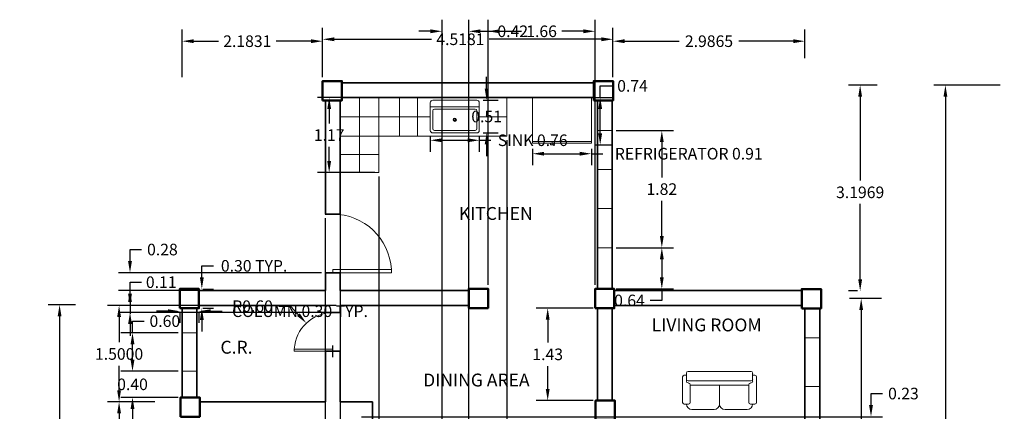
# Model space of a CAD drawing. Units: metres. Extents: x 473.2 to 488.6, y 701.8 to 717.3.
# Tile 4 of 4: x 473.3 to 488.6, y 711.3 to 717.3. Entities that reach past the tile are written whole.
import ezdxf

# ---------------------------------------------------------------- set-up
doc = ezdxf.new("R2010")
doc.units = ezdxf.units.M
doc.header["$PDMODE"] = 32
for name, color, linetype, lineweight in [('A-ANNO-DIMS', 2, 'Continuous', 18), ('A-AREA-IDEN', 7, 'Continuous', 18), ('A-COLS', 7, 'Continuous', 50), ('A-DOOR', 3, 'Continuous', 18), ('A-EQPM', 8, 'Continuous', 18), ('A-FLOR-CASE', 9, 'Continuous', 18), ('A-FLOR-FIXT', 9, 'Continuous', 18), ('A-FURN', 8, 'Continuous', 18), ('A-GLAZ', 4, 'Continuous', 18), ('A-WALL', 7, 'Continuous', 35)]:
    doc.layers.add(name, color=color, linetype=linetype, lineweight=lineweight)
doc.styles.get("Standard").update_dxf_attribs({"font": 'arial.ttf'})
doc.dimstyles.get("Standard").update_dxf_attribs({"dimtxt": 0.18, "dimasz": 0.18, "dimexe": 0.18, "dimexo": 0.0625, "dimgap": 0.09, "dimtad": 0, "dimtih": 1, "dimtoh": 1, "dimdec": 4, "dimzin": 0, "dimdsep": 46, "dimtxsty": 'Standard', "dimcen": 0.09, "dimadec": 0, "dimazin": 0, "dimtfac": 1, "dimtdec": 4, "dimtofl": 0, "dimtmove": 0, "dimatfit": 3, "dimfxl": 1, "dimtolj": 1, "dimtzin": 0, "dimarcsym": 0})

# ---------------------------------------------------------------- blocks, each defined once
blk = doc.blocks.new('A$C02A636C4')
for p, q in [((0, 0.572), (0, 0.126)), ((0.068, 0.601), (0.029, 0.601)), ((0.068, 0.64), (0.068, 0.601)), ((0.068, 0.533), (0.068, 0.601)), ((0.068, 0.495), (0.068, 0.543)), ((1.203, 0.669), (0.097, 0.669)), ((1.232, 0.64), (1.232, 0.601)), ((1.232, 0.601), (1.271, 0.601)), ((1.232, 0.533), (1.232, 0.601)), ((1.232, 0.495), (1.232, 0.543)), ((1.3, 0.572), (1.3, 0.126)), ((1.203, 0.504), (0.097, 0.504)), ((0.107, 0.466), (0.097, 0.466)), ((0.136, 0.126), (0.136, 0.436)), ((1.164, 0.427), (0.136, 0.427)), ((0.65, 0.097), (0.65, 0.427)), ((1.164, 0.126), (1.164, 0.436)), ((1.193, 0.466), (1.203, 0.466)), ((0.029, 0.097), (0.107, 0.097)), ((0.165, 0), (0.553, 0)), ((0.747, 0), (1.135, 0)), ((1.271, 0.097), (1.193, 0.097))]:
    blk.add_line(p, q)
for centre, radius, start, end in [((0.029, 0.572), 0.0291, 90, 180), ((0.097, 0.64), 0.0291, 90, 180), ((0.097, 0.533), 0.0291, 180, 270), ((1.203, 0.64), 0.0291, 0, 90), ((1.203, 0.533), 0.0291, 270, 0), ((1.271, 0.572), 0.0291, 0, 90), ((0.097, 0.495), 0.0291, 180, 270), ((0.107, 0.436), 0.0291, 0, 90), ((1.193, 0.436), 0.0291, 90, 180), ((1.203, 0.495), 0.0291, 270, 0), ((0.029, 0.126), 0.0291, 180, 270), ((0.165, 0.097), 0.097, 180, 270), ((0.107, 0.126), 0.0291, 270, 0), ((0.553, 0.097), 0.097, 270, 0), ((0.747, 0.097), 0.097, 180, 270), ((1.135, 0.097), 0.097, 270, 0), ((1.193, 0.126), 0.0291, 180, 270), ((1.271, 0.126), 0.0291, 270, 0)]:
    blk.add_arc(centre, radius, start, end)
blk = doc.blocks.new('Sink-single - 30 in top')
blk.add_line((-15, -3.999996), (15, -3.999996))
for points in [[(-13.5, 0), (13.5, 0)], [(-15, -18.499996), (-15, -1.5)], [(-12.5, -5.499996), (12.5, -5.499996)], [(15, -1.5), (15, -18.499996)], [(-13.5, -17.499996), (-13.5, -6.499996)], [(13.5, -6.499996), (13.5, -17.499996)], [(13.5, -19.999996), (-13.5, -19.999996)], [(12.5, -18.499996), (-12.5, -18.499996)]]:
    blk.add_lwpolyline(points)
for radius in [1, 0.5]:
    blk.add_circle((0, -11.999996), radius)
for centre, radius, start, end in [((-13.5, -1.5), 1.5, 90, 180), ((-12.5, -6.499996), 1, 90, 180), ((12.5, -6.499996), 1, 0, 90), ((13.5, -1.5), 1.5, 0, 90), ((-12.5, -17.499996), 1, 180, 270), ((12.5, -17.499996), 1, 270, 0), ((-13.5, -18.499996), 1.5, 180, 270), ((13.5, -18.499996), 1.5, 270, 0)]:
    blk.add_arc(centre, radius, start, end)
blk = doc.blocks.new('Refrigerator-2 door - 36 in top')
for p, q in [((0, -26.999999), (36, -26.999999)), ((11, -27.999999), (11, -28.999999)), ((11, -28.999999), (13, -28.999999)), ((12, -26.999999), (12, -28.999999)), ((13, -28.999999), (13, -27.999999))]:
    blk.add_line(p, q)
blk.add_lwpolyline([(0, -27.999999), (0, 0), (36, 0), (36, -27.999999)], close=True)
blk = doc.blocks.new('*D6')
at = {"layer": 'A-ANNO-DIMS', "color": 0, "lineweight": -2, "transparency": 16777216}
for p, q in [((482.501, 716.452), (482.501, 717.189)), ((485.488, 716.744), (485.488, 717.189)), ((482.681, 717.009), (483.529, 717.009)), ((485.308, 717.009), (484.461, 717.009))]:
    blk.add_line(p, q, dxfattribs=at)
at = {"layer": 'A-ANNO-DIMS', "color": 0, "transparency": 16777216}
for points in [[(482.681, 717.039), (482.681, 716.979), (482.501, 717.009)], [(485.308, 717.039), (485.308, 716.979), (485.488, 717.009)]]:
    blk.add_solid(points, dxfattribs=at)
at = {"layer": 'Defpoints', "color": 0, "transparency": 16777216}
for p in [(485.488, 717.009), (485.488, 716.681), (482.501, 716.39)]:
    blk.add_point(p, dxfattribs=at)
at = {"layer": 'A-ANNO-DIMS', "color": 0, "transparency": 16777216, "insert": (483.995, 717.009), "char_height": 0.18, "width": 1.24026, "attachment_point": 5}
blk.add_mtext('\\A1;2.9865', dxfattribs=at)
blk = doc.blocks.new('*D7')
at = {"layer": 'A-ANNO-DIMS', "color": 0, "lineweight": -2, "transparency": 16777216}
for p, q in [((477.983, 716.452), (477.983, 717.219)), ((482.501, 716.644), (482.501, 717.219)), ((478.163, 717.039), (479.677, 717.039)), ((482.321, 717.039), (480.577, 717.039))]:
    blk.add_line(p, q, dxfattribs=at)
at = {"layer": 'A-ANNO-DIMS', "color": 0, "transparency": 16777216}
for points in [[(478.163, 717.069), (478.163, 717.009), (477.983, 717.039)], [(482.321, 717.069), (482.321, 717.009), (482.501, 717.039)]]:
    blk.add_solid(points, dxfattribs=at)
at = {"layer": 'Defpoints', "color": 0, "transparency": 16777216}
for p in [(482.501, 717.039), (482.501, 716.581), (477.983, 716.39)]:
    blk.add_point(p, dxfattribs=at)
at = {"layer": 'A-ANNO-DIMS', "color": 0, "transparency": 16777216, "insert": (480.127, 717.039), "char_height": 0.18, "width": 1.24026, "attachment_point": 5}
blk.add_mtext('\\A1;4.5181', dxfattribs=at)
blk = doc.blocks.new('*D8')
at = {"layer": 'A-ANNO-DIMS', "color": 0, "lineweight": -2, "transparency": 16777216}
for p, q in [((475.798, 716.452), (475.798, 717.189)), ((477.981, 716.744), (477.981, 717.189)), ((475.978, 717.009), (476.363, 717.009)), ((477.801, 717.009), (477.259, 717.009))]:
    blk.add_line(p, q, dxfattribs=at)
at = {"layer": 'A-ANNO-DIMS', "color": 0, "transparency": 16777216}
for points in [[(475.978, 717.039), (475.978, 716.979), (475.798, 717.009)], [(477.801, 717.039), (477.801, 716.979), (477.981, 717.009)]]:
    blk.add_solid(points, dxfattribs=at)
at = {"layer": 'Defpoints', "color": 0, "transparency": 16777216}
for p in [(477.981, 717.009), (477.981, 716.681), (475.798, 716.39)]:
    blk.add_point(p, dxfattribs=at)
at = {"layer": 'A-ANNO-DIMS', "color": 0, "transparency": 16777216, "insert": (476.811, 717.009), "char_height": 0.18, "width": 1.24026, "attachment_point": 5}
blk.add_mtext('\\A1;2.1831', dxfattribs=at)
blk = doc.blocks.new('*D10')
at = {"layer": 'A-ANNO-DIMS', "color": 0, "lineweight": -2, "transparency": 16777216}
for p, q in [((475.082, 712.905), (474.636, 712.905)), ((474.816, 712.725), (474.816, 712.332)), ((474.816, 711.585), (474.816, 711.968)), ((475.373, 711.405), (474.636, 711.405))]:
    blk.add_line(p, q, dxfattribs=at)
at = {"layer": 'A-ANNO-DIMS', "color": 0, "transparency": 16777216}
for points in [[(474.786, 712.725), (474.846, 712.725), (474.816, 712.905)], [(474.786, 711.585), (474.846, 711.585), (474.816, 711.405)]]:
    blk.add_solid(points, dxfattribs=at)
at = {"layer": 'Defpoints', "color": 0, "transparency": 16777216}
for p in [(474.816, 712.905), (475.144, 712.905), (475.435, 711.405)]:
    blk.add_point(p, dxfattribs=at)
at = {"layer": 'A-ANNO-DIMS', "color": 0, "transparency": 16777216, "insert": (474.816, 712.15), "char_height": 0.18, "width": 1.24026, "attachment_point": 5}
blk.add_mtext('\\A1;1.5000', dxfattribs=at)
blk = doc.blocks.new('*D11')
at = {"layer": 'A-ANNO-DIMS', "color": 0, "lineweight": -2, "transparency": 16777216}
for p, q in [((475.082, 711.405), (474.636, 711.405)), ((474.816, 711.225), (474.816, 709.784)), ((474.816, 707.857), (474.816, 709.421)), ((475.373, 707.677), (474.636, 707.677))]:
    blk.add_line(p, q, dxfattribs=at)
at = {"layer": 'A-ANNO-DIMS', "color": 0, "transparency": 16777216}
for points in [[(474.786, 711.225), (474.846, 711.225), (474.816, 711.405)], [(474.786, 707.857), (474.846, 707.857), (474.816, 707.677)]]:
    blk.add_solid(points, dxfattribs=at)
at = {"layer": 'Defpoints', "color": 0, "transparency": 16777216}
for p in [(474.816, 711.405), (475.144, 711.405), (475.435, 707.677)]:
    blk.add_point(p, dxfattribs=at)
at = {"layer": 'A-ANNO-DIMS', "color": 0, "transparency": 16777216, "insert": (474.816, 709.602), "char_height": 0.18, "width": 1.24026, "attachment_point": 5}
blk.add_mtext('\\A1;3.7277', dxfattribs=at)
blk = doc.blocks.new('*D13')
at = {"layer": 'A-ANNO-DIMS', "color": 0, "lineweight": -2, "transparency": 16777216}
for p, q in [((474.139, 712.914), (473.71, 712.914)), ((473.89, 712.734), (473.89, 708.817)), ((473.89, 704.612), (473.89, 708.453)), ((473.889, 704.432), (473.71, 704.432))]:
    blk.add_line(p, q, dxfattribs=at)
at = {"layer": 'A-ANNO-DIMS', "color": 0, "transparency": 16777216}
for points in [[(473.86, 712.734), (473.92, 712.734), (473.89, 712.914)], [(473.86, 704.612), (473.92, 704.612), (473.89, 704.432)]]:
    blk.add_solid(points, dxfattribs=at)
at = {"layer": 'Defpoints', "color": 0, "transparency": 16777216}
for p in [(473.89, 712.914), (474.201, 712.914), (473.952, 704.432)]:
    blk.add_point(p, dxfattribs=at)
at = {"layer": 'A-ANNO-DIMS', "color": 0, "transparency": 16777216, "insert": (473.89, 708.635), "char_height": 0.18, "width": 1.24026, "attachment_point": 5}
blk.add_mtext('\\A1;8.4814', dxfattribs=at)
blk = doc.blocks.new('*D14')
at = {"layer": 'A-ANNO-DIMS', "color": 0, "lineweight": -2, "transparency": 16777216}
for p, q in [((486.68, 713.013), (486.183, 713.013)), ((486.363, 712.833), (486.363, 710.74)), ((486.363, 707.857), (486.363, 710.376)), ((486.92, 707.677), (486.183, 707.677))]:
    blk.add_line(p, q, dxfattribs=at)
at = {"layer": 'A-ANNO-DIMS', "color": 0, "transparency": 16777216}
for points in [[(486.333, 712.833), (486.393, 712.833), (486.363, 713.013)], [(486.333, 707.857), (486.393, 707.857), (486.363, 707.677)]]:
    blk.add_solid(points, dxfattribs=at)
at = {"layer": 'Defpoints', "color": 0, "transparency": 16777216}
for p in [(486.363, 713.013), (486.743, 713.013), (486.982, 707.677)]:
    blk.add_point(p, dxfattribs=at)
at = {"layer": 'A-ANNO-DIMS', "color": 0, "transparency": 16777216, "insert": (486.363, 710.558), "char_height": 0.18, "width": 1.24026, "attachment_point": 5}
blk.add_mtext('\\A1;5.3358', dxfattribs=at)
blk = doc.blocks.new('*D16')
at = {"layer": 'A-ANNO-DIMS', "color": 0, "lineweight": -2, "transparency": 16777216}
for p, q in [((486.612, 716.326), (486.167, 716.326)), ((486.347, 716.146), (486.347, 714.843)), ((486.347, 713.309), (486.347, 714.48)), ((486.308, 713.129), (486.167, 713.129))]:
    blk.add_line(p, q, dxfattribs=at)
at = {"layer": 'A-ANNO-DIMS', "color": 0, "transparency": 16777216}
for points in [[(486.317, 716.146), (486.377, 716.146), (486.347, 716.326)], [(486.317, 713.309), (486.377, 713.309), (486.347, 713.129)]]:
    blk.add_solid(points, dxfattribs=at)
at = {"layer": 'Defpoints', "color": 0, "transparency": 16777216}
for p in [(486.347, 716.326), (486.675, 716.326), (486.37, 713.129)]:
    blk.add_point(p, dxfattribs=at)
at = {"layer": 'A-ANNO-DIMS', "color": 0, "transparency": 16777216, "insert": (486.347, 714.661), "char_height": 0.18, "width": 1.24026, "attachment_point": 5}
blk.add_mtext('\\A1;3.1969', dxfattribs=at)
blk = doc.blocks.new('*D17')
at = {"layer": 'A-ANNO-DIMS', "color": 0, "lineweight": -2, "transparency": 16777216}
for p, q in [((488.527, 716.326), (487.494, 716.326)), ((487.674, 716.146), (487.674, 710.717)), ((487.674, 704.395), (487.674, 710.356)), ((488.223, 704.215), (487.494, 704.215))]:
    blk.add_line(p, q, dxfattribs=at)
at = {"layer": 'A-ANNO-DIMS', "color": 0, "transparency": 16777216}
for points in [[(487.644, 716.146), (487.704, 716.146), (487.674, 716.326)], [(487.644, 704.395), (487.704, 704.395), (487.674, 704.215)]]:
    blk.add_solid(points, dxfattribs=at)
at = {"layer": 'Defpoints', "color": 0, "transparency": 16777216}
for p in [(487.674, 716.326), (488.59, 716.326), (488.285, 704.215)]:
    blk.add_point(p, dxfattribs=at)
at = {"layer": 'A-ANNO-DIMS', "color": 0, "transparency": 16777216, "insert": (487.674, 710.536), "char_height": 0.18, "width": 1.24026, "attachment_point": 5}
blk.add_mtext('\\A1;12.1117', dxfattribs=at)
blk = doc.blocks.new('DOOR-SWING-910')
for p, q in [((0, 0), (-0.05, 0)), ((-0.05, 0), (-0.05, -0.91)), ((0, 0), (0, -0.91)), ((0, -0.91), (-0.05, -0.91))]:
    blk.add_line(p, q)
blk.add_arc((0.001, 0), 0.911, 180, 266.7638)
blk = doc.blocks.new('COL-SQUARE-300')
blk.add_lwpolyline([(-0.15, -0.15), (0.15, -0.15), (0.15, 0.15), (-0.15, 0.15)], close=True)
blk = doc.blocks.new('WIN-1520')
blk.add_line((0.23, 0.76), (0, 0.76))
blk.add_lwpolyline([(0.23, 0), (0.23, 1.52), (0, 1.52), (0, 0)], close=True)
blk = doc.blocks.new('*D25')
at = {"layer": 'A-ANNO-DIMS', "color": 0, "lineweight": -2, "transparency": 16777216}
for p, q in [((475.579, 712.814), (475.399, 712.814)), ((475.759, 712.797), (475.759, 712.634)), ((476.059, 712.797), (476.059, 712.634)), ((476.239, 712.814), (476.419, 712.814))]:
    blk.add_line(p, q, dxfattribs=at)
at = {"layer": 'A-ANNO-DIMS', "color": 0, "transparency": 16777216}
for points in [[(475.579, 712.844), (475.579, 712.784), (475.759, 712.814)], [(476.239, 712.844), (476.239, 712.784), (476.059, 712.814)]]:
    blk.add_solid(points, dxfattribs=at)
at = {"layer": 'Defpoints', "color": 0, "transparency": 16777216}
for p in [(475.759, 712.859), (476.059, 712.859), (476.059, 712.814)]:
    blk.add_point(p, dxfattribs=at)
at = {"layer": 'A-ANNO-DIMS', "color": 0, "transparency": 16777216, "insert": (477.631, 712.814), "char_height": 0.18, "attachment_point": 5}
blk.add_mtext('\\A1;COLUMN 0.30 TYP.', dxfattribs=at)
blk = doc.blocks.new('*D26')
at = {"layer": 'A-ANNO-DIMS', "color": 0, "lineweight": -2, "transparency": 16777216}
for p, q in [((476.104, 713.339), (476.104, 713.519)), ((476.104, 713.519), (476.284, 713.519)), ((476.121, 713.159), (476.284, 713.159)), ((476.121, 712.859), (476.284, 712.859)), ((476.104, 712.679), (476.104, 712.499))]:
    blk.add_line(p, q, dxfattribs=at)
at = {"layer": 'A-ANNO-DIMS', "color": 0, "transparency": 16777216}
for points in [[(476.074, 713.339), (476.134, 713.339), (476.104, 713.159)], [(476.074, 712.679), (476.134, 712.679), (476.104, 712.859)]]:
    blk.add_solid(points, dxfattribs=at)
at = {"layer": 'Defpoints', "color": 0, "transparency": 16777216}
for p in [(476.059, 713.159), (476.104, 713.159), (476.059, 712.859)]:
    blk.add_point(p, dxfattribs=at)
at = {"layer": 'A-ANNO-DIMS', "color": 0, "transparency": 16777216, "insert": (476.917, 713.519), "char_height": 0.18, "attachment_point": 5}
blk.add_mtext('\\A1;0.30 TYP.', dxfattribs=at)
blk = doc.blocks.new('*D39')
at = {"layer": 'A-ANNO-DIMS', "color": 0, "lineweight": -2, "transparency": 16777216}
for p, q in [((479.659, 715.522), (479.659, 715.29)), ((479.839, 715.47), (480.241, 715.47)), ((480.421, 715.522), (480.421, 715.29)), ((480.421, 715.47), (480.601, 715.47))]:
    blk.add_line(p, q, dxfattribs=at)
at = {"layer": 'A-ANNO-DIMS', "color": 0, "transparency": 16777216}
for points in [[(479.839, 715.5), (479.839, 715.44), (479.659, 715.47)], [(480.241, 715.5), (480.241, 715.44), (480.421, 715.47)]]:
    blk.add_solid(points, dxfattribs=at)
at = {"layer": 'Defpoints', "color": 0, "transparency": 16777216}
for p in [(479.659, 715.585), (480.421, 715.585), (480.421, 715.47)]:
    blk.add_point(p, dxfattribs=at)
at = {"layer": 'A-ANNO-DIMS', "color": 0, "transparency": 16777216, "insert": (481.252, 715.47), "char_height": 0.18, "attachment_point": 5}
blk.add_mtext('\\A1;SINK 0.76', dxfattribs=at)
blk = doc.blocks.new('*D40')
at = {"layer": 'A-ANNO-DIMS', "color": 0, "lineweight": -2, "transparency": 16777216}
for p, q in [((480.535, 716.273), (480.535, 716.453)), ((480.483, 716.093), (480.715, 716.093)), ((480.483, 715.585), (480.715, 715.585)), ((480.535, 715.405), (480.535, 715.225))]:
    blk.add_line(p, q, dxfattribs=at)
at = {"layer": 'A-ANNO-DIMS', "color": 0, "transparency": 16777216}
for points in [[(480.505, 716.273), (480.565, 716.273), (480.535, 716.093)], [(480.505, 715.405), (480.565, 715.405), (480.535, 715.585)]]:
    blk.add_solid(points, dxfattribs=at)
at = {"layer": 'Defpoints', "color": 0, "transparency": 16777216}
for p in [(480.421, 716.093), (480.535, 716.093), (480.421, 715.585)]:
    blk.add_point(p, dxfattribs=at)
at = {"layer": 'A-ANNO-DIMS', "color": 0, "transparency": 16777216, "insert": (480.535, 715.839), "char_height": 0.18, "attachment_point": 5}
blk.add_mtext('\\A1;0.51', dxfattribs=at)
blk = doc.blocks.new('*D41')
at = {"layer": 'A-ANNO-DIMS', "color": 0, "lineweight": -2, "transparency": 16777216}
for p, q in [((481.25, 715.335), (481.25, 715.081)), ((482.165, 715.335), (482.165, 715.081)), ((481.43, 715.261), (481.985, 715.261)), ((482.165, 715.261), (482.345, 715.261))]:
    blk.add_line(p, q, dxfattribs=at)
at = {"layer": 'A-ANNO-DIMS', "color": 0, "transparency": 16777216}
for points in [[(481.43, 715.291), (481.43, 715.231), (481.25, 715.261)], [(481.985, 715.291), (481.985, 715.231), (482.165, 715.261)]]:
    blk.add_solid(points, dxfattribs=at)
at = {"layer": 'Defpoints', "color": 0, "transparency": 16777216}
for p in [(481.25, 715.398), (482.165, 715.398), (482.165, 715.261)]:
    blk.add_point(p, dxfattribs=at)
at = {"layer": 'A-ANNO-DIMS', "color": 0, "transparency": 16777216, "insert": (483.68, 715.261), "char_height": 0.18, "attachment_point": 5}
blk.add_mtext('\\A1;REFRIGERATOR 0.91', dxfattribs=at)
blk = doc.blocks.new('*D42')
at = {"layer": 'A-ANNO-DIMS', "color": 0, "lineweight": -2, "transparency": 16777216}
for p, q in [((482.302, 716.135), (482.302, 716.315)), ((482.302, 716.315), (482.482, 716.315)), ((482.227, 716.135), (482.482, 716.135)), ((482.302, 715.578), (482.302, 715.955)), ((482.227, 715.398), (482.482, 715.398))]:
    blk.add_line(p, q, dxfattribs=at)
at = {"layer": 'A-ANNO-DIMS', "color": 0, "transparency": 16777216}
for points in [[(482.272, 715.955), (482.332, 715.955), (482.302, 716.135)], [(482.272, 715.578), (482.332, 715.578), (482.302, 715.398)]]:
    blk.add_solid(points, dxfattribs=at)
at = {"layer": 'Defpoints', "color": 0, "transparency": 16777216}
for p in [(482.165, 716.135), (482.302, 716.135), (482.165, 715.398)]:
    blk.add_point(p, dxfattribs=at)
at = {"layer": 'A-ANNO-DIMS', "color": 0, "transparency": 16777216, "insert": (482.805, 716.315), "char_height": 0.18, "attachment_point": 5}
blk.add_mtext('\\A1;0.74', dxfattribs=at)
blk = doc.blocks.new('*D44')
at = {"layer": 'A-ANNO-DIMS', "color": 0, "lineweight": -2, "transparency": 16777216}
for p, q in [((486.516, 711.355), (486.516, 711.535)), ((486.516, 711.535), (486.696, 711.535)), ((478.59, 711.175), (486.696, 711.175)), ((478.59, 710.948), (486.696, 710.948)), ((486.516, 710.768), (486.516, 710.588))]:
    blk.add_line(p, q, dxfattribs=at)
at = {"layer": 'A-ANNO-DIMS', "color": 0, "transparency": 16777216}
for points in [[(486.486, 711.355), (486.546, 711.355), (486.516, 711.175)], [(486.486, 710.768), (486.546, 710.768), (486.516, 710.948)]]:
    blk.add_solid(points, dxfattribs=at)
at = {"layer": 'Defpoints', "color": 0, "transparency": 16777216}
for p in [(478.528, 711.175), (486.516, 711.175), (478.528, 710.948)]:
    blk.add_point(p, dxfattribs=at)
at = {"layer": 'A-ANNO-DIMS', "color": 0, "transparency": 16777216, "insert": (487.02, 711.535), "char_height": 0.18, "attachment_point": 5}
blk.add_mtext('\\A1;0.23', dxfattribs=at)
blk = doc.blocks.new('*D45')
at = {"layer": 'A-ANNO-DIMS', "color": 0, "lineweight": -2, "transparency": 16777216}
for p, q in [((474.986, 713.085), (474.986, 713.265)), ((474.986, 713.265), (475.166, 713.265)), ((478.195, 712.905), (474.806, 712.905)), ((478.195, 712.794), (474.806, 712.794)), ((474.986, 712.614), (474.986, 712.434))]:
    blk.add_line(p, q, dxfattribs=at)
at = {"layer": 'A-ANNO-DIMS', "color": 0, "transparency": 16777216}
for points in [[(474.956, 713.085), (475.016, 713.085), (474.986, 712.905)], [(474.956, 712.614), (475.016, 712.614), (474.986, 712.794)]]:
    blk.add_solid(points, dxfattribs=at)
at = {"layer": 'Defpoints', "color": 0, "transparency": 16777216}
for p in [(474.986, 712.905), (478.258, 712.905), (478.258, 712.794)]:
    blk.add_point(p, dxfattribs=at)
at = {"layer": 'A-ANNO-DIMS', "color": 0, "transparency": 16777216, "insert": (475.472, 713.265), "char_height": 0.18, "attachment_point": 5}
blk.add_mtext('\\A1;0.11', dxfattribs=at)
blk = doc.blocks.new('*D46')
at = {"layer": 'A-ANNO-DIMS', "color": 0, "lineweight": -2, "transparency": 16777216}
for p, q in [((474.986, 713.592), (474.986, 713.772)), ((474.986, 713.772), (475.166, 713.772)), ((477.965, 713.412), (474.806, 713.412)), ((477.965, 713.135), (474.806, 713.135)), ((474.986, 712.955), (474.986, 712.775))]:
    blk.add_line(p, q, dxfattribs=at)
at = {"layer": 'A-ANNO-DIMS', "color": 0, "transparency": 16777216}
for points in [[(474.956, 713.592), (475.016, 713.592), (474.986, 713.412)], [(474.956, 712.955), (475.016, 712.955), (474.986, 713.135)]]:
    blk.add_solid(points, dxfattribs=at)
at = {"layer": 'Defpoints', "color": 0, "transparency": 16777216}
for p in [(474.986, 713.412), (478.028, 713.412), (478.028, 713.135)]:
    blk.add_point(p, dxfattribs=at)
at = {"layer": 'A-ANNO-DIMS', "color": 0, "transparency": 16777216, "insert": (475.49, 713.772), "char_height": 0.18, "attachment_point": 5}
blk.add_mtext('\\A1;0.28', dxfattribs=at)
blk = doc.blocks.new('*D47')
at = {"layer": 'A-ANNO-DIMS', "color": 0, "lineweight": -2, "transparency": 16777216}
for p, q in [((480.558, 713.226), (480.558, 717.343)), ((482.222, 713.223), (482.222, 717.343)), ((480.738, 717.163), (481.075, 717.163)), ((482.042, 717.163), (481.705, 717.163))]:
    blk.add_line(p, q, dxfattribs=at)
at = {"layer": 'A-ANNO-DIMS', "color": 0, "transparency": 16777216}
for points in [[(480.738, 717.193), (480.738, 717.133), (480.558, 717.163)], [(482.042, 717.193), (482.042, 717.133), (482.222, 717.163)]]:
    blk.add_solid(points, dxfattribs=at)
at = {"layer": 'Defpoints', "color": 0, "transparency": 16777216}
for p in [(482.222, 717.163), (480.558, 713.164), (482.222, 713.161)]:
    blk.add_point(p, dxfattribs=at)
at = {"layer": 'A-ANNO-DIMS', "color": 0, "transparency": 16777216, "insert": (481.39, 717.163), "char_height": 0.18, "attachment_point": 5}
blk.add_mtext('\\A1;1.66', dxfattribs=at)
blk = doc.blocks.new('*D48')
at = {"layer": 'A-ANNO-DIMS', "color": 0, "lineweight": -2, "transparency": 16777216}
for p, q in [((482.195, 712.861), (481.305, 712.861)), ((481.485, 712.681), (481.485, 712.326)), ((481.485, 711.608), (481.485, 711.962)), ((482.195, 711.428), (481.305, 711.428))]:
    blk.add_line(p, q, dxfattribs=at)
at = {"layer": 'A-ANNO-DIMS', "color": 0, "transparency": 16777216}
for points in [[(481.455, 712.681), (481.515, 712.681), (481.485, 712.861)], [(481.455, 711.608), (481.515, 711.608), (481.485, 711.428)]]:
    blk.add_solid(points, dxfattribs=at)
at = {"layer": 'Defpoints', "color": 0, "transparency": 16777216}
for p in [(481.485, 712.861), (482.258, 712.861), (482.258, 711.428)]:
    blk.add_point(p, dxfattribs=at)
at = {"layer": 'A-ANNO-DIMS', "color": 0, "transparency": 16777216, "insert": (481.485, 712.144), "char_height": 0.18, "attachment_point": 5}
blk.add_mtext('\\A1;1.43', dxfattribs=at)
blk = doc.blocks.new('*D50')
at = {"layer": 'A-ANNO-DIMS', "color": 0, "lineweight": -2, "transparency": 16777216}
for p, q in [((479.841, 707.737), (479.841, 717.343)), ((480.258, 707.737), (480.258, 717.343)), ((479.661, 717.163), (479.481, 717.163)), ((480.438, 717.163), (480.618, 717.163))]:
    blk.add_line(p, q, dxfattribs=at)
at = {"layer": 'A-ANNO-DIMS', "color": 0, "transparency": 16777216}
for points in [[(479.661, 717.193), (479.661, 717.133), (479.841, 717.163)], [(480.438, 717.193), (480.438, 717.133), (480.258, 717.163)]]:
    blk.add_solid(points, dxfattribs=at)
at = {"layer": 'Defpoints', "color": 0, "transparency": 16777216}
for p in [(480.258, 717.163), (479.841, 707.675), (480.258, 707.675)]:
    blk.add_point(p, dxfattribs=at)
at = {"layer": 'A-ANNO-DIMS', "color": 0, "transparency": 16777216, "insert": (480.941, 717.163), "char_height": 0.18, "attachment_point": 5}
blk.add_mtext('\\A1;0.42', dxfattribs=at)
blk = doc.blocks.new('*D54')
at = {"layer": 'A-ANNO-DIMS', "color": 0, "lineweight": -2, "transparency": 16777216}
for p, q in [((478.024, 714.259), (478.024, 703.22)), ((478.258, 714.259), (478.258, 703.22)), ((477.844, 703.4), (477.664, 703.4)), ((478.438, 703.4), (478.618, 703.4))]:
    blk.add_line(p, q, dxfattribs=at)
at = {"layer": 'A-ANNO-DIMS', "color": 0, "transparency": 16777216}
for points in [[(477.844, 703.43), (477.844, 703.37), (478.024, 703.4)], [(478.438, 703.43), (478.438, 703.37), (478.258, 703.4)]]:
    blk.add_solid(points, dxfattribs=at)
at = {"layer": 'Defpoints', "color": 0, "transparency": 16777216}
for p in [(478.024, 714.322), (478.258, 714.322), (478.258, 703.4)]:
    blk.add_point(p, dxfattribs=at)
at = {"layer": 'A-ANNO-DIMS', "color": 0, "transparency": 16777216, "insert": (478.942, 703.4), "char_height": 0.18, "attachment_point": 5}
blk.add_mtext('\\A1;0.23', dxfattribs=at)
blk = doc.blocks.new('*D58')
at = {"layer": 'A-ANNO-DIMS', "color": 0, "lineweight": -2, "transparency": 16777216}
for p, q in [((482.55, 713.801), (483.441, 713.801)), ((483.261, 713.621), (483.261, 713.341)), ((482.55, 713.161), (483.441, 713.161)), ((483.261, 713.161), (483.261, 712.981)), ((483.261, 712.981), (483.081, 712.981))]:
    blk.add_line(p, q, dxfattribs=at)
at = {"layer": 'A-ANNO-DIMS', "color": 0, "transparency": 16777216}
for points in [[(483.231, 713.621), (483.291, 713.621), (483.261, 713.801)], [(483.231, 713.341), (483.291, 713.341), (483.261, 713.161)]]:
    blk.add_solid(points, dxfattribs=at)
at = {"layer": 'Defpoints', "color": 0, "transparency": 16777216}
for p in [(482.488, 713.801), (482.488, 713.161), (483.261, 713.161)]:
    blk.add_point(p, dxfattribs=at)
at = {"layer": 'A-ANNO-DIMS', "color": 0, "transparency": 16777216, "insert": (482.758, 712.981), "char_height": 0.18, "attachment_point": 5}
blk.add_mtext('\\A1;0.64', dxfattribs=at)
blk = doc.blocks.new('*D59')
at = {"layer": 'A-ANNO-DIMS', "color": 0, "lineweight": -2, "transparency": 16777216}
for p, q in [((482.55, 715.621), (483.441, 715.621)), ((483.261, 715.441), (483.261, 714.893)), ((483.261, 713.981), (483.261, 714.529)), ((482.55, 713.801), (483.441, 713.801))]:
    blk.add_line(p, q, dxfattribs=at)
at = {"layer": 'A-ANNO-DIMS', "color": 0, "transparency": 16777216}
for points in [[(483.231, 715.441), (483.291, 715.441), (483.261, 715.621)], [(483.231, 713.981), (483.291, 713.981), (483.261, 713.801)]]:
    blk.add_solid(points, dxfattribs=at)
at = {"layer": 'Defpoints', "color": 0, "transparency": 16777216}
for p in [(482.488, 715.621), (482.488, 713.801), (483.261, 713.801)]:
    blk.add_point(p, dxfattribs=at)
at = {"layer": 'A-ANNO-DIMS', "color": 0, "transparency": 16777216, "insert": (483.261, 714.711), "char_height": 0.18, "attachment_point": 5}
blk.add_mtext('\\A1;1.82', dxfattribs=at)
blk = doc.blocks.new('*D60')
at = {"layer": 'A-ANNO-DIMS', "color": 0, "lineweight": -2, "transparency": 16777216}
for p, q in [((475.025, 712.06), (475.025, 712.24)), ((475.735, 711.88), (474.845, 711.88)), ((475.735, 711.475), (474.845, 711.475)), ((475.025, 711.295), (475.025, 711.115))]:
    blk.add_line(p, q, dxfattribs=at)
at = {"layer": 'A-ANNO-DIMS', "color": 0, "transparency": 16777216}
for points in [[(474.995, 712.06), (475.055, 712.06), (475.025, 711.88)], [(474.995, 711.295), (475.055, 711.295), (475.025, 711.475)]]:
    blk.add_solid(points, dxfattribs=at)
at = {"layer": 'Defpoints', "color": 0, "transparency": 16777216}
for p in [(475.025, 711.88), (475.798, 711.88), (475.798, 711.475)]:
    blk.add_point(p, dxfattribs=at)
at = {"layer": 'A-ANNO-DIMS', "color": 0, "transparency": 16777216, "insert": (475.025, 711.678), "char_height": 0.18, "attachment_point": 5}
blk.add_mtext('\\A1;0.40', dxfattribs=at)
blk = doc.blocks.new('*D61')
at = {"layer": 'A-ANNO-DIMS', "color": 0, "lineweight": -2, "transparency": 16777216}
for p, q in [((475.025, 712.48), (475.025, 712.66)), ((475.025, 712.66), (475.205, 712.66)), ((475.735, 712.48), (474.845, 712.48)), ((475.025, 712.06), (475.025, 712.3)), ((475.735, 711.88), (474.845, 711.88))]:
    blk.add_line(p, q, dxfattribs=at)
at = {"layer": 'A-ANNO-DIMS', "color": 0, "transparency": 16777216}
for points in [[(474.995, 712.3), (475.055, 712.3), (475.025, 712.48)], [(474.995, 712.06), (475.055, 712.06), (475.025, 711.88)]]:
    blk.add_solid(points, dxfattribs=at)
at = {"layer": 'Defpoints', "color": 0, "transparency": 16777216}
for p in [(475.025, 712.48), (475.798, 712.48), (475.798, 711.88)]:
    blk.add_point(p, dxfattribs=at)
at = {"layer": 'A-ANNO-DIMS', "color": 0, "transparency": 16777216, "insert": (475.528, 712.66), "char_height": 0.18, "attachment_point": 5}
blk.add_mtext('\\A1;0.60', dxfattribs=at)
blk = doc.blocks.new('*D64')
at = {"layer": 'A-ANNO-DIMS', "color": 0, "lineweight": -2, "transparency": 16777216}
for p, q in [((478.258, 715.472), (478.258, 703.22)), ((480.85, 715.472), (480.85, 703.22)), ((478.438, 703.4), (479.228, 703.4)), ((480.67, 703.4), (479.879, 703.4))]:
    blk.add_line(p, q, dxfattribs=at)
at = {"layer": 'A-ANNO-DIMS', "color": 0, "transparency": 16777216}
for points in [[(478.438, 703.43), (478.438, 703.37), (478.258, 703.4)], [(480.67, 703.43), (480.67, 703.37), (480.85, 703.4)]]:
    blk.add_solid(points, dxfattribs=at)
at = {"layer": 'Defpoints', "color": 0, "transparency": 16777216}
for p in [(478.258, 715.535), (480.85, 715.535), (480.85, 703.4)]:
    blk.add_point(p, dxfattribs=at)
at = {"layer": 'A-ANNO-DIMS', "color": 0, "transparency": 16777216, "insert": (479.554, 703.4), "char_height": 0.18, "attachment_point": 5}
blk.add_mtext('\\A1;2.59', dxfattribs=at)
blk = doc.blocks.new('*D65')
at = {"layer": 'A-ANNO-DIMS', "color": 0, "lineweight": -2, "transparency": 16777216}
for p, q in [((478.795, 716.135), (477.905, 716.135)), ((478.085, 715.955), (478.085, 715.731)), ((478.085, 715.147), (478.085, 715.37)), ((478.795, 714.967), (477.905, 714.967))]:
    blk.add_line(p, q, dxfattribs=at)
at = {"layer": 'A-ANNO-DIMS', "color": 0, "transparency": 16777216}
for points in [[(478.055, 715.955), (478.115, 715.955), (478.085, 716.135)], [(478.055, 715.147), (478.115, 715.147), (478.085, 714.967)]]:
    blk.add_solid(points, dxfattribs=at)
at = {"layer": 'Defpoints', "color": 0, "transparency": 16777216}
for p in [(478.085, 716.135), (478.858, 716.135), (478.858, 714.967)]:
    blk.add_point(p, dxfattribs=at)
at = {"layer": 'A-ANNO-DIMS', "color": 0, "transparency": 16777216, "insert": (478.085, 715.551), "char_height": 0.18, "attachment_point": 5}
blk.add_mtext('\\A1;1.17', dxfattribs=at)
blk = doc.blocks.new('*D66')
at = {"layer": 'A-ANNO-DIMS', "color": 0, "lineweight": -2, "transparency": 16777216}
for p, q in [((478.258, 714.905), (478.258, 703.22)), ((478.858, 714.905), (478.858, 703.22)), ((478.438, 703.4), (478.678, 703.4)), ((478.858, 703.4), (479.038, 703.4))]:
    blk.add_line(p, q, dxfattribs=at)
at = {"layer": 'A-ANNO-DIMS', "color": 0, "transparency": 16777216}
for points in [[(478.438, 703.43), (478.438, 703.37), (478.258, 703.4)], [(478.678, 703.43), (478.678, 703.37), (478.858, 703.4)]]:
    blk.add_solid(points, dxfattribs=at)
at = {"layer": 'Defpoints', "color": 0, "transparency": 16777216}
for p in [(478.258, 714.967), (478.858, 714.967), (478.858, 703.4)]:
    blk.add_point(p, dxfattribs=at)
at = {"layer": 'A-ANNO-DIMS', "color": 0, "transparency": 16777216, "insert": (479.361, 703.4), "char_height": 0.18, "attachment_point": 5}
blk.add_mtext('\\A1;0.60', dxfattribs=at)
blk = doc.blocks.new('*D67')
at = {"layer": 'A-ANNO-DIMS', "color": 0, "lineweight": -2, "transparency": 16777216}
for p, q in [((477.302, 712.892), (477.482, 712.892)), ((477.482, 712.892), (477.606, 712.76)), ((478.143, 712.102), (478.143, 712.282)), ((478.053, 712.192), (478.233, 712.192))]:
    blk.add_line(p, q, dxfattribs=at)
at = {"layer": 'A-ANNO-DIMS', "color": 0, "transparency": 16777216}
blk.add_solid([(477.628, 712.781), (477.584, 712.74), (477.73, 712.629)], dxfattribs=at)
at = {"layer": 'Defpoints', "color": 0, "transparency": 16777216}
for p in [(477.73, 712.629), (478.143, 712.192)]:
    blk.add_point(p, dxfattribs=at)
at = {"layer": 'A-ANNO-DIMS', "color": 0, "transparency": 16777216, "insert": (476.892, 712.892), "char_height": 0.18, "attachment_point": 5}
blk.add_mtext('\\A1;R0.60', dxfattribs=at)

msp = doc.modelspace()

# ---------------------------------------------------------------- linework, layer by layer
at = {"layer": 'A-DOOR'}
for p, q in [((478.14297, 712.22584), (477.54211, 712.22584)), ((477.54211, 712.19283), (477.54211, 712.22584)), ((478.14297, 712.19283), (477.54211, 712.19283)), ((478.14297, 712.19283), (478.14297, 712.22584))]:
    msp.add_line(p, q, dxfattribs=at)
msp.add_arc((478.14297, 712.19187), 0.60182, 90, 176.763811, dxfattribs=at)
at = {"layer": 'A-FLOR-CASE'}
for p, q in [((478.55797, 714.9671), (478.55797, 716.13456)), ((478.85797, 715.53456), (478.85797, 716.13456)), ((479.17931, 715.53456), (479.17931, 716.13456)), ((479.46103, 715.53456), (479.46103, 716.13456)), ((480.56, 716.13456), (480.56, 715.53456)), ((480.84954, 716.13456), (480.84954, 715.53456)), ((479.65871, 715.83456), (478.25797, 715.83456)), ((480.84954, 715.83456), (480.42071, 715.83456)), ((478.85797, 715.53456), (478.25797, 715.53456)), ((478.85797, 715.53456), (480.84954, 715.53456)), ((478.85797, 714.9671), (478.85797, 715.53456)), ((478.85797, 715.25083), (478.25797, 715.25083)), ((478.85797, 714.9671), (478.25797, 714.9671))]:
    msp.add_line(p, q, dxfattribs=at)
at = {"layer": 'A-GLAZ'}
for p, q in [((482.25797, 715.62097), (482.48797, 715.62097)), ((482.25797, 715.0143), (482.48797, 715.0143)), ((482.25797, 714.40763), (482.48797, 714.40763)), ((482.48797, 713.80097), (482.25797, 713.80097))]:
    msp.add_line(p, q, dxfattribs=at)
msp.add_lwpolyline([(475.79797, 711.88009), (476.02797, 711.88009), (476.02797, 712.48009), (475.79797, 712.48009)], close=True, dxfattribs=at)
at = {"layer": 'A-WALL'}
for p, q in [((478.28334, 716.36456), (482.20148, 716.36456)), ((478.02797, 714.32196), (478.02797, 716.08968)), ((478.25797, 714.31468), (478.25797, 716.08968)), ((478.28334, 716.13456), (482.20148, 716.13456)), ((482.25797, 713.16085), (482.25797, 716.08968)), ((482.48797, 713.16085), (482.48797, 716.08968)), ((478.25797, 714.32196), (478.02407, 714.32196)), ((478.02797, 713.13456), (478.02797, 713.41196)), ((478.25797, 713.41196), (478.02797, 713.41196)), ((478.02797, 713.41196), (478.02797, 713.33995)), ((478.25797, 713.13456), (478.25797, 713.41196)), ((476.05887, 713.13456), (478.02797, 713.13456)), ((478.25797, 713.13456), (480.25797, 713.13456)), ((480.25797, 713.13456), (480.25797, 712.90456)), ((482.52164, 713.13456), (485.43907, 713.13456)), ((475.79797, 711.47539), (475.79797, 712.85934)), ((476.02797, 711.47539), (476.02797, 712.85934)), ((476.05887, 712.90456), (478.02797, 712.90456)), ((478.02797, 712.7826), (478.02797, 712.90456)), ((478.25797, 712.90456), (480.25797, 712.90456)), ((478.25797, 712.79369), (478.25797, 712.90456)), ((482.25797, 711.42764), (482.25797, 712.86085)), ((482.48797, 711.42764), (482.48797, 712.86085)), ((482.52164, 712.90456), (485.43907, 712.90456)), ((478.25797, 712.79369), (478.02797, 712.79369)), ((485.48797, 707.71527), (485.48797, 712.85771)), ((485.71797, 707.71527), (485.71797, 712.85771)), ((478.02797, 711.40456), (478.02797, 712.19369)), ((478.25797, 712.19283), (478.02797, 712.19283)), ((478.25797, 711.40456), (478.25797, 712.19369)), ((476.07166, 711.40456), (478.02797, 711.40456)), ((478.25797, 711.40456), (478.75797, 711.40456)), ((478.75797, 710.94776), (478.75797, 711.40456)), ((482.48797, 711.42764), (482.25797, 711.42764))]:
    msp.add_line(p, q, dxfattribs=at)

# ---------------------------------------------------------------- block references
at = {"layer": 'A-COLS'}
for p in [(478.13334, 716.23968), (482.35148, 716.23968), (475.90887, 713.00934), (480.40797, 713.01391), (482.37164, 713.01085), (485.58907, 713.00771), (475.92166, 711.32539), (482.38113, 711.27646)]:
    msp.add_blockref('COL-SQUARE-300', p, dxfattribs=at)
at = {"layer": 'A-DOOR', "extrusion": (0, 0, -1), "zscale": -1, "rotation": 269.999999999987}
msp.add_blockref('DOOR-SWING-910', (-478.14297, 713.41196), dxfattribs=at)
at = {"layer": 'A-EQPM', "xscale": 0.0254, "yscale": 0.0254, "zscale": 0.0254}
msp.add_blockref('Refrigerator-2 door - 36 in top', (481.25021, 716.13456), dxfattribs=at)
at = {"layer": 'A-FLOR-FIXT', "xscale": 0.0254, "yscale": 0.0254, "zscale": 0.0254}
msp.add_blockref('Sink-single - 30 in top', (480.03971, 716.09259), dxfattribs=at)
at = {"layer": 'A-FURN', "xscale": 0.8851373679523337, "yscale": 0.8851373679523337, "zscale": 0.8851373679523337}
msp.add_blockref('A$C02A636C4', (483.58388, 711.28654), dxfattribs=at)
at = {"layer": 'A-GLAZ'}
msp.add_blockref('WIN-1520', (485.48797, 710.88205), dxfattribs=at)

# ---------------------------------------------------------------- texts
at = {"layer": 'A-AREA-IDEN', "char_height": 0.2, "attachment_point": 1}
for s, insert in [('KITCHEN', (480.10189, 714.43255)), ('LIVING ROOM', (483.1032, 712.70096)), ('C.R.', (476.39301, 712.35444)), ('DINING AREA', (479.54686, 711.84468))]:
    msp.add_mtext_dynamic_manual_height_columns(s, width=2.8211562, gutter_width=12.5, heights=[0], dxfattribs=dict(at, insert=insert))

# ---------------------------------------------------------------- dimensions: what is measured, and where the dimension line sits
at = {"layer": 'A-ANNO-DIMS'}
for base, p1, p2, picture, middle in [((480.25797, 717.16268), (479.84132, 707.67456), (480.25797, 707.67456), '*D50', (480.94083, 717.16268)), ((482.22164, 717.16268), (480.55797, 713.16391), (482.22164, 713.16085), '*D47', (481.38981, 717.16268)), ((480.84954, 703.3995), (478.25797, 715.53456), (480.84954, 715.53456), '*D64', (479.55376, 703.3995)), ((478.85797, 703.3995), (478.25797, 714.9671), (478.85797, 714.9671), '*D66', (479.36144, 703.3995)), ((478.25797, 703.3995), (478.02407, 714.32196), (478.25797, 714.32196), '*D54', (478.94175, 703.3995))]:
    dim = msp.add_linear_dim(base=base, p1=p1, p2=p2, dimstyle='Standard', override={"dimdec": 2, "dimlfac": 1, "dimrnd": 0, "dimzin": 0, "dimdsep": 46, "dimlunit": 2}, dxfattribs=at)
    dim.commit()
    dim.dimension.update_dxf_attribs({"geometry": picture, "text_midpoint": middle})
for base, p1, p2, picture, middle in [((477.98103, 717.00882), (475.79797, 716.38968), (477.98103, 716.68107), '*D8', (476.8112, 717.00882)), ((482.50148, 717.03882), (477.98334, 716.38968), (482.50148, 716.58124), '*D7', (480.12676, 717.03882)), ((485.48797, 717.00882), (482.50148, 716.38968), (485.48797, 716.68107), '*D6', (483.99473, 717.00882))]:
    dim = msp.add_linear_dim(base=base, p1=p1, p2=p2, dimstyle='Standard', override={"dimclrd": 0, "dimclre": 0, "dimclrt": 0}, dxfattribs=at)
    dim.commit()
    dim.dimension.update_dxf_attribs({"geometry": picture, "text_midpoint": middle, "dimtype": 160})
for base, p1, p2, angle, picture, middle in [((480.53501, 716.09259), (480.42071, 715.58459), (480.42071, 716.09259), 90, '*D40', (480.53501, 715.83859)), ((482.30177, 716.13456), (482.16461, 715.39796), (482.16461, 716.13456), 90, '*D42', (482.80518, 716.31456)), ((478.08497, 716.13456), (478.85797, 714.9671), (478.85797, 716.13456), 90, '*D65', (478.08497, 715.55083)), ((483.26097, 713.80097), (482.48797, 715.62097), (482.48797, 713.80097), 270, '*D59', (483.26097, 714.71097)), ((474.98588, 713.41196), (478.02797, 713.13456), (478.02797, 713.41196), 90, '*D46', (475.48984, 713.77196)), ((483.26097, 713.16085), (482.48797, 713.80097), (482.48797, 713.16085), 270, '*D58', (482.75756, 712.98085)), ((474.98588, 712.90456), (478.25797, 712.79369), (478.25797, 712.90456), 90, '*D45', (475.47228, 713.26456)), ((481.48497, 712.86085), (482.25797, 711.42764), (482.25797, 712.86085), 90, '*D48', (481.48497, 712.14424)), ((475.02497, 712.48009), (475.79797, 711.88009), (475.79797, 712.48009), 90, '*D61', (475.52844, 712.66009)), ((475.02497, 711.88009), (475.79797, 711.47539), (475.79797, 711.88009), 90, '*D60', (475.02497, 711.67774)), ((486.51584, 711.17456), (478.52797, 710.94776), (478.52797, 711.17456), 90, '*D44', (487.01962, 711.53456))]:
    dim = msp.add_linear_dim(base=base, p1=p1, p2=p2, angle=angle, dimstyle='Standard', override={"dimdec": 2, "dimlfac": 1, "dimrnd": 0, "dimzin": 0, "dimdsep": 46, "dimlunit": 2}, dxfattribs=at)
    dim.commit()
    dim.dimension.update_dxf_attribs({"geometry": picture, "text_midpoint": middle})
for base, p1, p2, picture, middle in [((486.3472, 716.32625), (486.37025, 713.12937), (486.67495, 716.32625), '*D16', (486.3472, 714.66147)), ((487.67367, 716.32625), (488.28524, 704.21456), (488.58994, 716.32625), '*D17', (487.67367, 710.53618)), ((486.36295, 713.01265), (486.98209, 707.67682), (486.74295, 713.01265), '*D14', (486.36295, 710.55792)), ((473.88966, 712.91383), (473.95159, 704.4324), (474.20147, 712.91383), '*D13', (473.88966, 708.63485)), ((474.81629, 712.90456), (475.43544, 711.40456), (475.14404, 712.90456), '*D10', (474.81629, 712.14983)), ((474.81629, 711.40456), (475.43544, 707.67682), (475.14404, 711.40456), '*D11', (474.81629, 709.60247))]:
    dim = msp.add_linear_dim(base=base, p1=p1, p2=p2, angle=90, dimstyle='Standard', override={"dimclrd": 0, "dimclre": 0, "dimclrt": 0}, dxfattribs=at)
    dim.commit()
    dim.dimension.update_dxf_attribs({"geometry": picture, "text_midpoint": middle, "dimtype": 160})
for base, p1, p2, text, picture, middle in [((480.42071, 715.47029), (479.65871, 715.58459), (480.42071, 715.58459), 'SINK <>', '*D39', (481.25238, 715.47029)), ((482.16461, 715.2608), (481.25021, 715.39796), (482.16461, 715.39796), 'REFRIGERATOR <>', '*D41', (483.68018, 715.2608)), ((476.05887, 712.81434), (475.75887, 712.85934), (476.05887, 712.85934), 'COLUMN <> TYP.', '*D25', (477.63056, 712.81434))]:
    dim = msp.add_linear_dim(base=base, p1=p1, p2=p2, text=text, dimstyle='Standard', override={"dimdec": 2, "dimlfac": 1, "dimrnd": 0, "dimzin": 0, "dimdsep": 46, "dimlunit": 2}, dxfattribs=at)
    dim.commit()
    dim.dimension.update_dxf_attribs({"geometry": picture, "text_midpoint": middle})
dim = msp.add_linear_dim(base=(476.10387, 713.15934), p1=(476.05887, 712.85934), p2=(476.05887, 713.15934), angle=90, text='<> TYP.', dimstyle='Standard', override={"dimdec": 2, "dimlfac": 1, "dimrnd": 0, "dimzin": 0, "dimdsep": 46, "dimlunit": 2}, dxfattribs=at)
dim.commit()
dim.dimension.update_dxf_attribs({"geometry": '*D26', "text_midpoint": (476.91682, 713.51934)})
dim = msp.add_radius_dim(center=(478.14297, 712.19187), mpoint=(477.72968, 712.62934), dimstyle='Standard', override={"dimdec": 2, "dimlfac": 1, "dimrnd": 0, "dimzin": 0, "dimdsep": 46, "dimlunit": 2}, dxfattribs=at)
dim.commit()
dim.dimension.update_dxf_attribs({"geometry": '*D67', "text_midpoint": (476.8921, 712.89182), "dimtype": 164})

doc.saveas('drawing.dxf')
